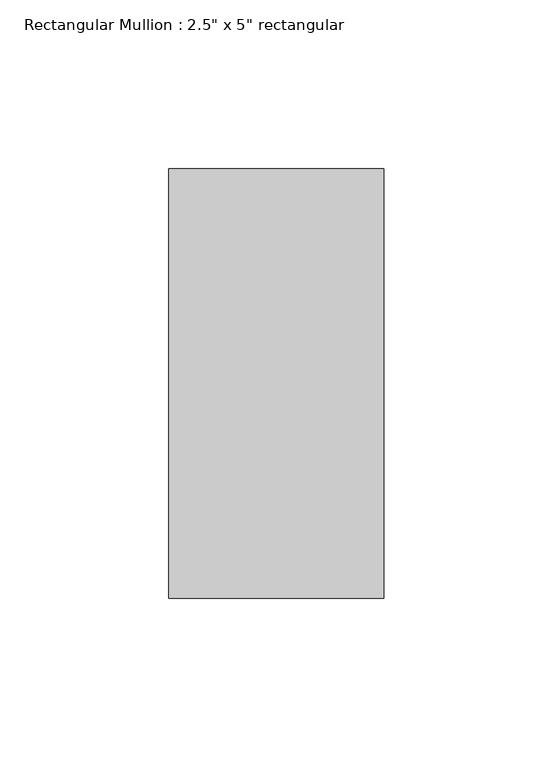
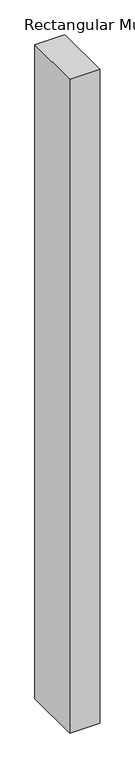
"""IFC4 building model written with IfcOpenShell, lengths in millimetres: member geometry."""

from ifc_helpers import new_model, si_unit, frame, origin, place, context, project, spatial, polyline, outline, extrude, source, transform, mapped, element, save


def member_19b327e1(model_context):
    return source(origin(), model_context, "Body", "SweptSolid", [
        extrude(outline(polyline([(0.0, 63.5), (0.0, -63.5), (-63.5, -63.5), (-63.5, 63.5), (0.0, 63.5)])), frame((0.0, 0.0, -1460.4999998), z_axis=(0.0, 0.0, 1.0), x_axis=(1.0, 0.0, 0.0)), (0.0, 0.0, 1.0), 1460.4999998),
    ])


if __name__ == "__main__":
    model = new_model("IFC4")
    model_context = context("Model", 3, world=origin())
    ifc_project = project(units=[si_unit("LENGTHUNIT", "METRE", prefix="MILLI")], contexts=[model_context])
    site = spatial("IfcSite", under=ifc_project)
    building = spatial("IfcBuilding", under=site)
    placement = place(None, origin())
    member_shape = member_19b327e1(model_context)
    element("IfcMember", 1, ObjectType="Rectangular Mullion : 2.5\" x 5\" rectangular", at=placement, inside=building, context=model_context, shape_type="MappedRepresentation", body=[
        mapped(member_shape, transform((0.0, 0.0, 0.0), x_axis=(1.0, 0.0, 0.0), y_axis=(0.0, 1.0, 0.0), z_axis=(0.0, 0.0, 1.0))),
    ])
    save(model, "model.ifc")

# Revit data of these elements
# Type "Rectangular Mullion : 2.5\" x 5\" rectangular"
#   built-in parameter 1007304 = 0.416667 (stored number, unit not read)
#   built-in parameter 1007301 = 0.104167 (stored number, unit not read)
#   built-in parameter 1007300 = 0.104167 (stored number, unit not read)
# Element 1 (IfcMember, "Rectangular Mullion : 2.5\" x 5\" rectangular")
#   Materials on its faces: "BLACK COLOUR"
# Materials
#   "BLACK COLOUR": class "Generic", colour RGB 120 120 120, transparency 0, Cost = 0
